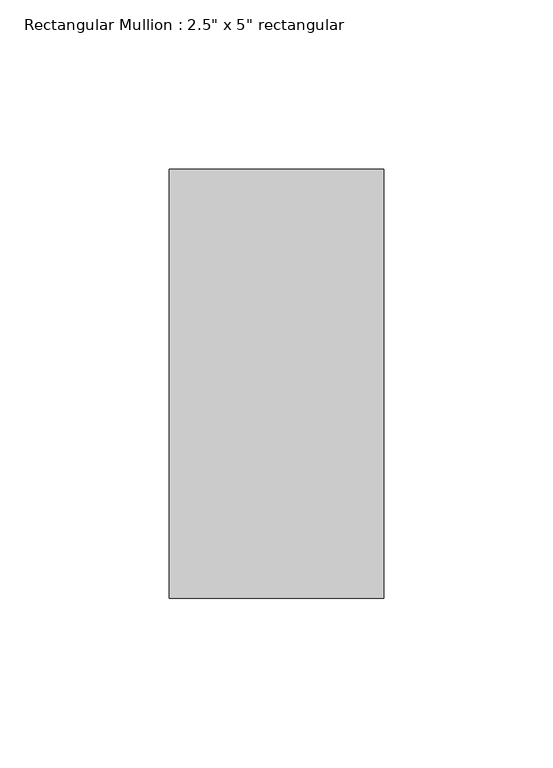
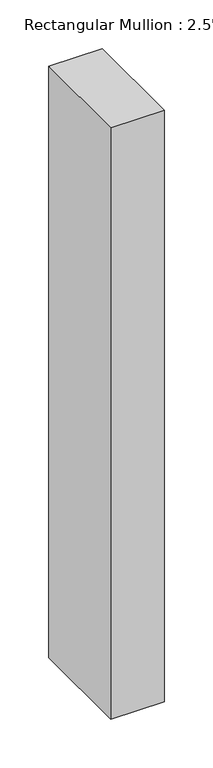
"""IFC4 building model written with IfcOpenShell, lengths in millimetres: member geometry."""

from ifc_helpers import new_model, si_unit, frame, origin, place, context, project, spatial, polyline, outline, extrude, source, transform, mapped, element, save


def member_0492494d(model_context):
    return source(origin(), model_context, "Body", "SweptSolid", [
        extrude(outline(polyline([(31.75, 63.5), (31.75, -63.5), (-31.75, -63.5), (-31.75, 63.5), (31.75, 63.5)])), frame((0.0, 0.0, -741.4158453), z_axis=(0.0, 0.0, 1.0), x_axis=(1.0, 0.0, 0.0)), (0.0, 0.0, 1.0), 741.4158453),
    ])


if __name__ == "__main__":
    model = new_model("IFC4")
    model_context = context("Model", 3, world=origin())
    ifc_project = project(units=[si_unit("LENGTHUNIT", "METRE", prefix="MILLI")], contexts=[model_context])
    site = spatial("IfcSite", under=ifc_project)
    building = spatial("IfcBuilding", under=site)
    placement = place(None, origin())
    member_shape = member_0492494d(model_context)
    element("IfcMember", 1, ObjectType="Rectangular Mullion : 2.5\" x 5\" rectangular", at=placement, inside=building, context=model_context, shape_type="MappedRepresentation", body=[
        mapped(member_shape, transform((0.0, 0.0, 0.0), x_axis=(1.0, 0.0, 0.0), y_axis=(0.0, 1.0, 0.0), z_axis=(0.0, 0.0, 1.0))),
    ])
    save(model, "model.ifc")

# Revit data of these elements
# Type "Rectangular Mullion : 2.5\" x 5\" rectangular"
#   built-in parameter 1007304 = 0.416667 (stored number, unit not read)
#   built-in parameter 1007301 = 0.104167 (stored number, unit not read)
#   built-in parameter 1007300 = 0.104167 (stored number, unit not read)
# Element 1 (IfcMember, "Rectangular Mullion : 2.5\" x 5\" rectangular")
#   Materials on its faces: "Aluminum"
# Materials
#   "Aluminum": class "Metal", colour RGB 247 247 247, transparency 0, Description = "Aluminum 6061", Cost = 0
